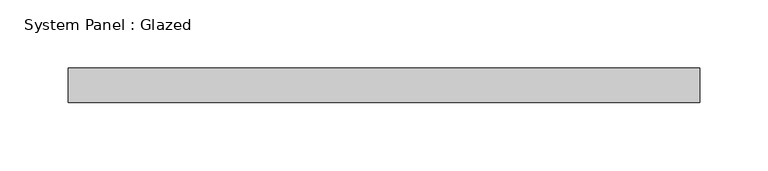
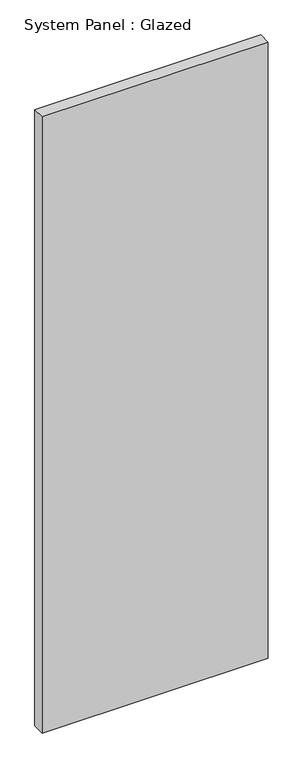
"""IFC4 building model written with IfcOpenShell, lengths in millimetres: plate geometry, System Panel : Glazed."""

from ifc_helpers import new_model, si_unit, origin, origin_with_axes, place, context, project, spatial, polyline, outline, extrude, source, transform, mapped, element, save


def system_panel_glazed_3f13655f(model_context):
    return source(origin(), model_context, "Body", "SweptSolid", [
        extrude(outline(polyline([(231.775, 19.05), (-231.775, 19.05), (-231.775, 44.45), (231.775, 44.45), (231.775, 19.05)])), origin_with_axes(), (0.0, 0.0, 1.0), 1335.4986146),
    ])


if __name__ == "__main__":
    model = new_model("IFC4")
    model_context = context("Model", 3, world=origin())
    ifc_project = project(units=[si_unit("LENGTHUNIT", "METRE", prefix="MILLI")], contexts=[model_context])
    site = spatial("IfcSite", under=ifc_project)
    building = spatial("IfcBuilding", under=site)
    placement = place(None, origin())
    system_panel_glazed_shape = system_panel_glazed_3f13655f(model_context)
    element("IfcPlate", 1, ObjectType="System Panel : Glazed", at=placement, inside=building, context=model_context, shape_type="MappedRepresentation", body=[
        mapped(system_panel_glazed_shape, transform((0.0, 0.0, 0.0), x_axis=(1.0, 0.0, 0.0), y_axis=(0.0, 1.0, 0.0), z_axis=(0.0, 0.0, 1.0))),
    ])
    save(model, "model.ifc")

# Revit data of these elements
# Type "System Panel : Glazed"
#   Construction Type Id = "GSP4R"
#   Analytic Construction = "1/8 in Pilkington single glazing"
#   Visual Light Transmittance = 0.9
#   Solar Heat Gain Coefficient = 0.86
#   Heat Transfer Coefficient (U) = 1.18115 BTU/(h·ft²·°F)
#   Define Thermal Properties by = 1
# Element 1 (IfcPlate, "System Panel : Glazed")
#   Materials on its faces: "Glass"
# Materials
#   "Glass": class "Glass", colour RGB 0 128 192, transparency 0.75, Description = "Soda Lime Glass", Cost = 0
